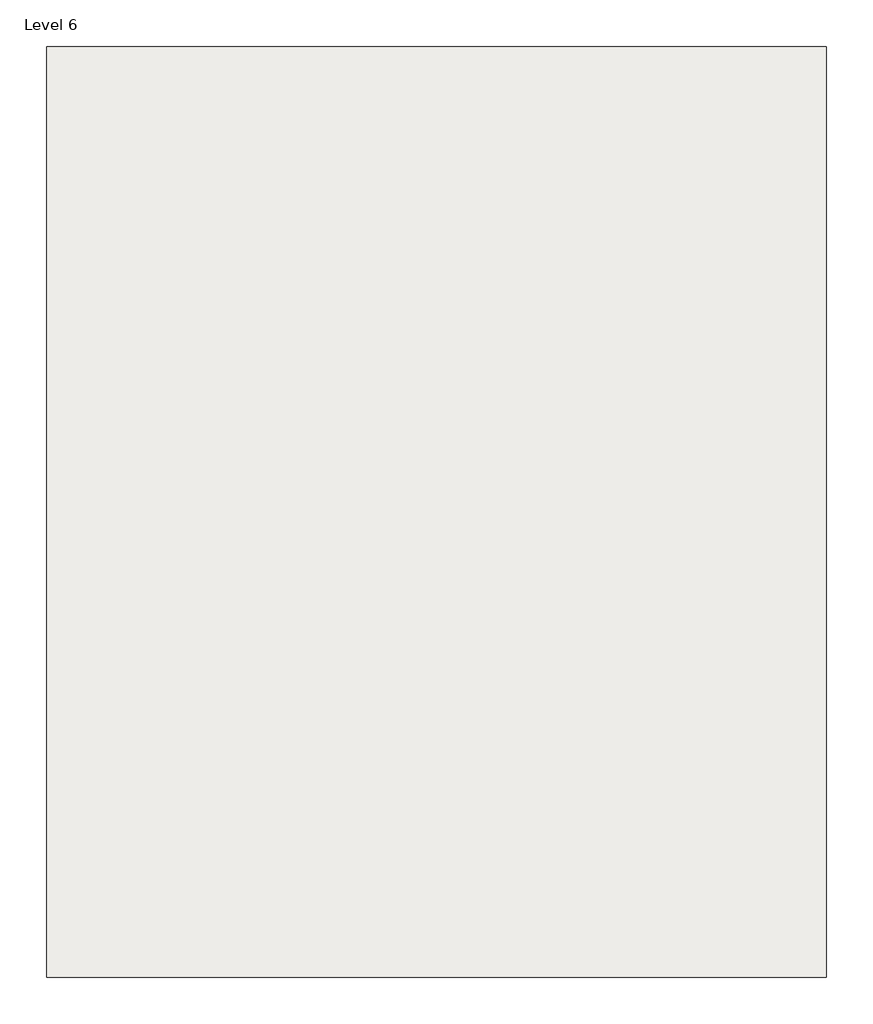
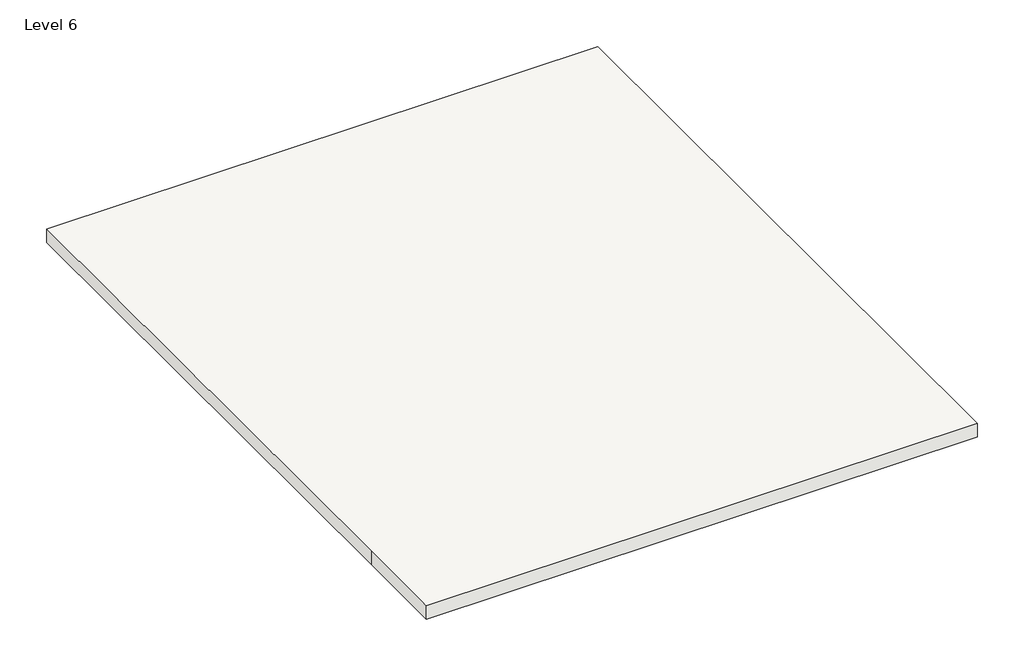
# One storey: 1 roof.
"""IFC4 building model written with IfcOpenShell, lengths in millimetres."""

from ifc_helpers import new_model, si_unit, frame, origin, place, context, project, spatial, polyline, outline, extrude, element, save

model = new_model("IFC4")

# Units and contexts
model_context = context("Model", 3, world=origin())
ifc_project = project(units=[si_unit("LENGTHUNIT", "METRE", prefix="MILLI")], contexts=[model_context])

# Site, building, storey
site = spatial("IfcSite", under=ifc_project)
building = spatial("IfcBuilding", under=site)
storey = spatial("IfcBuildingStorey", under=building, Name="Level 6", Elevation=18288.0)

# Roof
placement = place(None, origin())
element("IfcRoof", 1, ObjectType="Generic - 12\"", at=placement, inside=storey, context=model_context, shape_type="SweptSolid", body=[
    extrude(outline(polyline([(-8860.5727738, 10082.3674246), (2924.6563456, 10082.3674246), (2924.6563456, -3989.2325754), (-8860.5727738, -3989.2325754), (-8860.5727738, -1957.2325754), (-8860.5727738, 10082.3674246)])), frame((0.0, 0.0, 18288.0), z_axis=(0.0, 0.0, 1.0), x_axis=(1.0, 0.0, 0.0)), (0.0, 0.0, 1.0), 304.8),
])

save(model, "model.ifc")

# Revit data of these elements
# Type "Generic - 12\""
#   Assembly Code = "B1020"
#   Layers, outside or top first: 1' - 0" no material (function 1)
# Element 1 (IfcRoof, "Generic - 12\"")
#   built-in parameter 1001705 = 61 (stored number, unit not read)
#   built-in parameter 1001710 = 33615
#   Phase Created = New Construction
#   Materials on its faces: "Default Roof"
# Materials
#   "Default Roof": colour RGB 88 101 114, transparency 0
